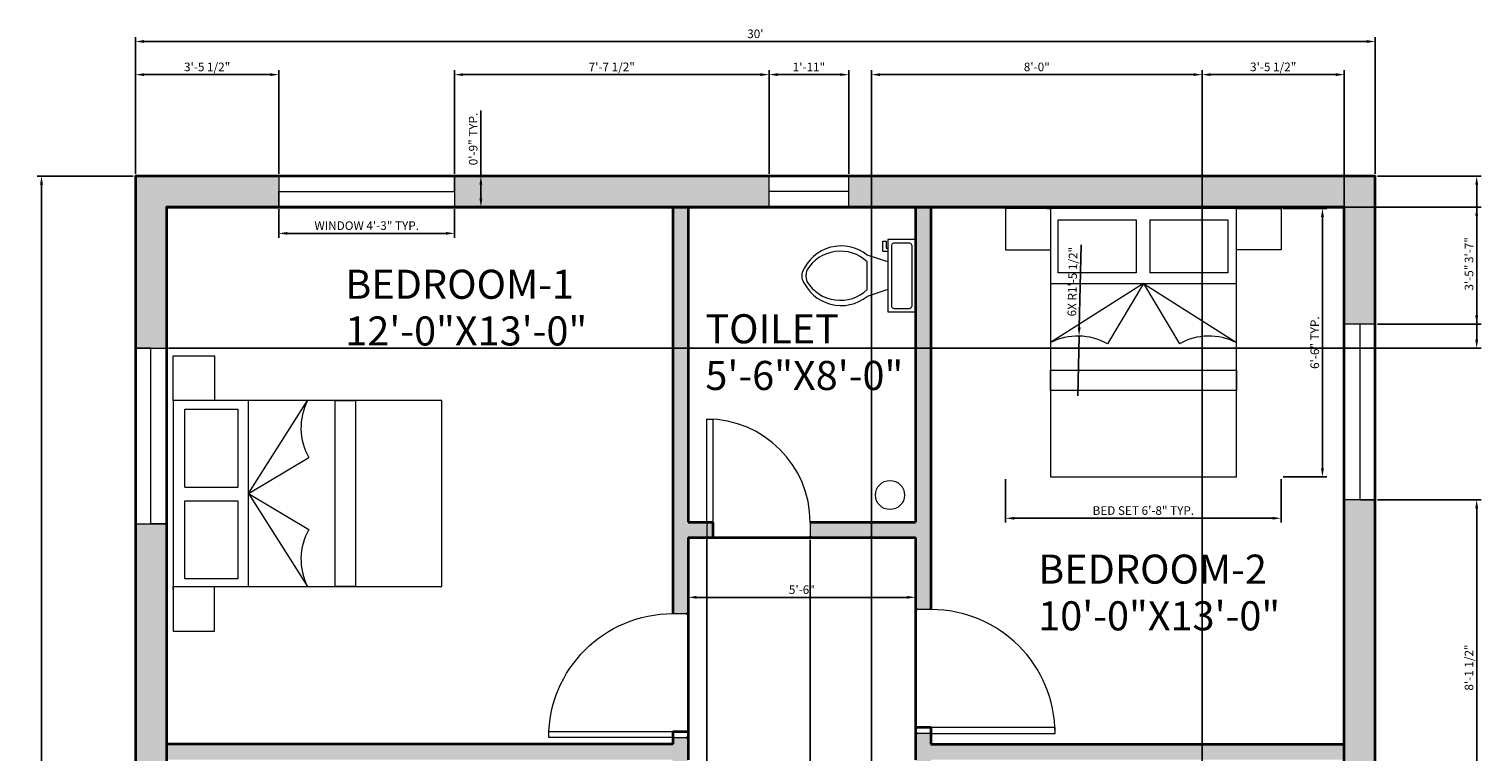
# Model space of a CAD drawing. Units: inches. Extents: x 10 to 434, y 91 to 681.
# Tile 2 of 2: x 12 to 434, y 471 to 681. Entities that reach past the tile are written whole.
import ezdxf

# ---------------------------------------------------------------- set-up
doc = ezdxf.new("R2010")
doc.units = ezdxf.units.IN
for name, color, linetype, lineweight in [('A-ANNO-DIMS', 2, 'Continuous', 18), ('A-AREA-IDEN', 7, 'Continuous', 18), ('A-DOOR', 4, 'Continuous', 18), ('A-FLOR-FIXT', 9, 'Continuous', 18), ('A-FURN', 8, 'Continuous', 18), ('A-GLAZ', 4, 'Continuous', 18), ('A-WALL', 7, 'Continuous', 35), ('A-WALL-PATT', 251, 'Continuous', 13)]:
    doc.layers.add(name, color=color, linetype=linetype, lineweight=lineweight)
doc.styles.get("Standard").update_dxf_attribs({"font": 'arial.ttf'})
doc.dimstyles.new('ISO-25', dxfattribs={"dimtxt": 2.5, "dimasz": 2.5, "dimexe": 1.25, "dimexo": 0.625, "dimtad": 1, "dimlunit": 3, "dimtxsty": 'Standard', "dimcen": 2.5, "dimadec": 0, "dimazin": 0, "dimtfac": 1, "dimtmove": 0, "dimatfit": 3, "dimfxl": 1, "dimarcsym": 0})

# ---------------------------------------------------------------- blocks, each defined once
blk = doc.blocks.new('*U4')
for p, q in [((0, 0), (0, -4)), ((-36, 0), (-36, -4))]:
    blk.add_line(p, q)
blk.add_lwpolyline([(0, 0), (0, 36), (-1.75, 36), (-1.75, 0)], close=True)
blk.add_arc((0, 0), 36, 90, 180)
blk = doc.blocks.new('*U3')
for p, q in [((0, 0), (0, -4)), ((30, 0), (30, -4))]:
    blk.add_line(p, q)
blk.add_lwpolyline([(0, 0), (0, 30), (1.75, 30), (1.75, 0)], close=True)
blk.add_arc((0, 0), 30, 0, 90)
blk = doc.blocks.new('*U7')
for p, q in [((9.5, -6), (9.5, -2)), ((-8, -8.5), (-8, -8)), ((-7, -8), (-7, -9.5)), ((-4, -8), (-6, -14)), ((4, -8), (6, -14)), ((-10, -8.5), (-8, -8.5)), ((-10, -9.5), (-10, -8.5)), ((-7, -9.5), (-10, -9.5)), ((4, -14), (-4, -14))]:
    blk.add_line(p, q)
blk.add_lwpolyline([(10.5, -8), (10.5, 0), (-10.5, 0), (-10.5, -8)], close=True)
for points in [[(-9.5, -2), (-9.5, -6)], [(8.5, -1), (-8.5, -1)], [(-8.5, -7), (8.5, -7)]]:
    blk.add_lwpolyline(points)
for centre, radius, start, end in [((-8.62, -1.88), 0.884, 81.8699, 188.1301), ((8.62, -1.88), 0.884, 351.8699, 98.1301), ((-8.62, -6.12), 0.884, 171.8699, 278.1301), ((8.62, -6.12), 0.884, 261.8699, 8.1301), ((3.52, -21.58), 12.17, 141.4691, 247.9714), ((4.2, -21.82), 11.33, 136.3677, 238.9468), ((-3.52, -21.58), 12.17, 292.0284, 38.5307), ((-4.2, -21.82), 11.33, 301.053, 43.6321), ((0, -27.88), 4, 245.7318, 294.2682), ((0, -29), 4, 254.8605, 285.1395)]:
    blk.add_arc(centre, radius, start, end)
blk = doc.blocks.new('*D11')
at = {"layer": 'A-ANNO-DIMS', "color": 0, "lineweight": -2, "transparency": 16777216}
for p, q in [((42.44, 638.74), (14.54, 638.74)), ((15.79, 636.24), (15.79, 161.24)), ((42.44, 158.74), (14.54, 158.74))]:
    blk.add_line(p, q, dxfattribs=at)
at = {"layer": 'A-ANNO-DIMS', "color": 0, "transparency": 16777216}
for points in [[(15.37, 636.24), (16.21, 636.24), (15.79, 638.74)], [(15.37, 161.24), (16.21, 161.24), (15.79, 158.74)]]:
    blk.add_solid(points, dxfattribs=at)
at = {"layer": 'Defpoints', "color": 0, "transparency": 16777216}
for p in [(43.07, 638.74), (15.79, 158.74), (43.07, 158.74)]:
    blk.add_point(p, dxfattribs=at)
at = {"layer": 'A-ANNO-DIMS', "color": 0, "transparency": 16777216, "insert": (13.89, 398.74), "char_height": 2.5, "attachment_point": 5, "rotation": 90}
blk.add_mtext("40'", dxfattribs=at)
blk = doc.blocks.new('*D12')
at = {"layer": 'A-ANNO-DIMS', "color": 0, "lineweight": -2, "transparency": 16777216}
for p, q in [((43.07, 639.37), (43.07, 679.06)), ((400.57, 677.81), (45.57, 677.81)), ((403.07, 639.37), (403.07, 679.06))]:
    blk.add_line(p, q, dxfattribs=at)
at = {"layer": 'A-ANNO-DIMS', "color": 0, "transparency": 16777216}
for points in [[(45.57, 678.23), (45.57, 677.4), (43.07, 677.81)], [(400.57, 678.23), (400.57, 677.4), (403.07, 677.81)]]:
    blk.add_solid(points, dxfattribs=at)
at = {"layer": 'Defpoints', "color": 0, "transparency": 16777216}
for p in [(43.07, 677.81), (43.07, 638.74), (403.07, 638.74)]:
    blk.add_point(p, dxfattribs=at)
at = {"layer": 'A-ANNO-DIMS', "color": 0, "transparency": 16777216, "insert": (223.07, 679.72), "char_height": 2.5, "attachment_point": 5}
blk.add_mtext("30'", dxfattribs=at)
blk = doc.blocks.new('*D14')
at = {"layer": 'A-ANNO-DIMS', "color": 0, "lineweight": -2, "transparency": 16777216}
for p, q in [((203.57, 533.12), (203.57, 515.14)), ((269.57, 533.12), (269.57, 515.14)), ((206.07, 516.39), (267.07, 516.39))]:
    blk.add_line(p, q, dxfattribs=at)
at = {"layer": 'A-ANNO-DIMS', "color": 0, "transparency": 16777216}
for points in [[(206.07, 516.81), (206.07, 515.98), (203.57, 516.39)], [(267.07, 516.81), (267.07, 515.98), (269.57, 516.39)]]:
    blk.add_solid(points, dxfattribs=at)
at = {"layer": 'Defpoints', "color": 0, "transparency": 16777216}
for p in [(203.57, 533.74), (269.57, 533.74), (269.57, 516.39)]:
    blk.add_point(p, dxfattribs=at)
at = {"layer": 'A-ANNO-DIMS', "color": 0, "transparency": 16777216, "insert": (236.57, 518.29), "char_height": 2.5, "attachment_point": 5}
blk.add_mtext('5\'-6"', dxfattribs=at)
blk = doc.blocks.new('BED-DOUBLE-WITH-NIGHTSTANDS')
for p, q in [((40, 21.85), (13, 39)), ((40, 21.85), (29.54, 39.37)), ((40, 21.85), (50.46, 39.37)), ((40, 21.85), (67, 39)), ((67, 21.85), (13, 21.85)), ((38.13, 3.34), (38.13, 18.76)), ((42.13, 3.34), (42.13, 18.76)), ((0, 0), (0, 12)), ((0, 12), (13, 12)), ((68, 12), (67, 12)), ((80, 12), (68, 12)), ((80, 0), (80, 12)), ((1, 0), (0, 0)), ((13, 0), (1, 0)), ((68, 0), (80, 0))]:
    blk.add_line(p, q)
for points in [[(67, 78), (13, 78), (13, 0), (67, 0)], [(67, 46.98), (13, 46.98), (13, 52.9), (67, 52.9)], [(67, 0), (68, 0), (68, 0), (67, 0)]]:
    blk.add_lwpolyline(points, close=True)
for points in [[(38.13, 3.34), (15.5, 3.34), (15.5, 18.76), (38.13, 18.76)], [(42.13, 18.76), (64.76, 18.76), (64.76, 3.34), (42.13, 3.34)]]:
    blk.add_lwpolyline(points)
for centre, start, end in [((20.93, 54.43), 242.8058, 299.7512), ((59.07, 54.43), 240.2488, 297.1942)]:
    blk.add_arc(centre, 17.35, start, end)
blk = doc.blocks.new('WINDOW-51IN')
for p, q in [((0, 9), (0, 0)), ((51, 4.5), (51, 9)), ((51, 9), (51, 0)), ((0, 0), (0, 4.5)), ((0, 4.5), (51, 4.5))]:
    blk.add_line(p, q)
blk = doc.blocks.new('*D20')
at = {"layer": 'A-ANNO-DIMS', "color": 0, "lineweight": -2, "transparency": 16777216}
for p, q in [((84.72, 629.12), (84.72, 620.84)), ((135.72, 629.12), (135.72, 620.84)), ((87.22, 622.09), (133.22, 622.09))]:
    blk.add_line(p, q, dxfattribs=at)
at = {"layer": 'A-ANNO-DIMS', "color": 0, "transparency": 16777216}
for points in [[(87.22, 622.51), (87.22, 621.68), (84.72, 622.09)], [(133.22, 622.51), (133.22, 621.68), (135.72, 622.09)]]:
    blk.add_solid(points, dxfattribs=at)
at = {"layer": 'Defpoints', "color": 0, "transparency": 16777216}
for p in [(84.72, 629.74), (135.72, 629.74), (135.72, 622.09)]:
    blk.add_point(p, dxfattribs=at)
at = {"layer": 'A-ANNO-DIMS', "color": 0, "transparency": 16777216, "insert": (110.22, 624.01), "char_height": 2.5, "attachment_point": 5}
blk.add_mtext('WINDOW 4\'-3" TYP.', dxfattribs=at)
blk = doc.blocks.new('*D21')
at = {"layer": 'A-ANNO-DIMS', "color": 0, "lineweight": -2, "transparency": 16777216}
for p, q in [((143.37, 638.74), (143.37, 657.73)), ((136.34, 638.74), (144.62, 638.74)), ((143.37, 632.24), (143.37, 636.24)), ((136.34, 629.74), (144.62, 629.74))]:
    blk.add_line(p, q, dxfattribs=at)
at = {"layer": 'A-ANNO-DIMS', "color": 0, "transparency": 16777216}
for points in [[(142.95, 636.24), (143.78, 636.24), (143.37, 638.74)], [(142.95, 632.24), (143.78, 632.24), (143.37, 629.74)]]:
    blk.add_solid(points, dxfattribs=at)
at = {"layer": 'Defpoints', "color": 0, "transparency": 16777216}
for p in [(135.72, 638.74), (143.37, 638.74), (135.72, 629.74)]:
    blk.add_point(p, dxfattribs=at)
at = {"layer": 'A-ANNO-DIMS', "color": 0, "transparency": 16777216, "insert": (141.46, 649.49), "char_height": 2.5, "attachment_point": 5, "rotation": 90}
blk.add_mtext('0\'-9" TYP.', dxfattribs=at)
blk = doc.blocks.new('*D22')
at = {"layer": 'A-ANNO-DIMS', "color": 0, "lineweight": -2, "transparency": 16777216}
for p, q in [((295.73, 550.73), (295.73, 538.1)), ((375.73, 550.73), (375.73, 538.1)), ((373.23, 539.35), (298.23, 539.35))]:
    blk.add_line(p, q, dxfattribs=at)
at = {"layer": 'A-ANNO-DIMS', "color": 0, "transparency": 16777216}
for points in [[(298.23, 539.77), (298.23, 538.94), (295.73, 539.35)], [(373.23, 539.77), (373.23, 538.94), (375.73, 539.35)]]:
    blk.add_solid(points, dxfattribs=at)
at = {"layer": 'Defpoints', "color": 0, "transparency": 16777216}
for p in [(295.73, 551.35), (375.73, 551.35), (295.73, 539.35)]:
    blk.add_point(p, dxfattribs=at)
at = {"layer": 'A-ANNO-DIMS', "color": 0, "transparency": 16777216, "insert": (335.73, 541.27), "char_height": 2.5, "attachment_point": 5}
blk.add_mtext('BED SET 6\'-8" TYP.', dxfattribs=at)
blk = doc.blocks.new('*D23')
at = {"layer": 'A-ANNO-DIMS', "color": 0, "lineweight": -2, "transparency": 16777216}
for p, q in [((376.36, 629.35), (388.98, 629.35)), ((387.73, 626.85), (387.73, 553.85)), ((376.36, 551.35), (388.98, 551.35))]:
    blk.add_line(p, q, dxfattribs=at)
at = {"layer": 'A-ANNO-DIMS', "color": 0, "transparency": 16777216}
for points in [[(387.31, 626.85), (388.15, 626.85), (387.73, 629.35)], [(387.31, 553.85), (388.15, 553.85), (387.73, 551.35)]]:
    blk.add_solid(points, dxfattribs=at)
at = {"layer": 'Defpoints', "color": 0, "transparency": 16777216}
for p in [(375.73, 629.35), (375.73, 551.35), (387.73, 551.35)]:
    blk.add_point(p, dxfattribs=at)
at = {"layer": 'A-ANNO-DIMS', "color": 0, "transparency": 16777216, "insert": (385.83, 590.35), "char_height": 2.5, "attachment_point": 5, "rotation": 90}
blk.add_mtext('6\'-6" TYP.', dxfattribs=at)
blk = doc.blocks.new('*D27')
at = {"layer": 'A-ANNO-DIMS', "color": 0, "lineweight": -2, "transparency": 16777216}
for p, q in [((352.79, 283.87), (352.79, 669.44)), ((355.29, 668.19), (391.57, 668.19)), ((394.07, 283.87), (394.07, 669.44))]:
    blk.add_line(p, q, dxfattribs=at)
at = {"layer": 'A-ANNO-DIMS', "color": 0, "transparency": 16777216}
for points in [[(355.29, 668.61), (355.29, 667.78), (352.79, 668.19)], [(391.57, 668.61), (391.57, 667.78), (394.07, 668.19)]]:
    blk.add_solid(points, dxfattribs=at)
at = {"layer": 'Defpoints', "color": 0, "transparency": 16777216}
for p in [(394.07, 668.19), (352.79, 283.24), (394.07, 283.24)]:
    blk.add_point(p, dxfattribs=at)
at = {"layer": 'A-ANNO-DIMS', "color": 0, "transparency": 16777216, "insert": (373.43, 670.11), "char_height": 2.5, "attachment_point": 5}
blk.add_mtext('3\'-5 1/2"', dxfattribs=at)
blk = doc.blocks.new('*D28')
at = {"layer": 'A-ANNO-DIMS', "color": 0, "lineweight": -2, "transparency": 16777216}
for p, q in [((256.79, 283.87), (256.79, 669.44)), ((259.29, 668.19), (350.29, 668.19)), ((352.79, 283.87), (352.79, 669.44))]:
    blk.add_line(p, q, dxfattribs=at)
at = {"layer": 'A-ANNO-DIMS', "color": 0, "transparency": 16777216}
for points in [[(259.29, 668.61), (259.29, 667.78), (256.79, 668.19)], [(350.29, 668.61), (350.29, 667.78), (352.79, 668.19)]]:
    blk.add_solid(points, dxfattribs=at)
at = {"layer": 'Defpoints', "color": 0, "transparency": 16777216}
for p in [(352.79, 668.19), (256.79, 283.24), (352.79, 283.24)]:
    blk.add_point(p, dxfattribs=at)
at = {"layer": 'A-ANNO-DIMS', "color": 0, "transparency": 16777216, "insert": (304.79, 670.1), "char_height": 2.5, "attachment_point": 5}
blk.add_mtext('8\'-0"', dxfattribs=at)
blk = doc.blocks.new('*D29')
at = {"layer": 'A-ANNO-DIMS', "color": 0, "lineweight": -2, "transparency": 16777216}
for p, q in [((43.07, 639.37), (43.07, 669.44)), ((45.57, 668.19), (82.22, 668.19)), ((84.72, 639.37), (84.72, 669.44))]:
    blk.add_line(p, q, dxfattribs=at)
at = {"layer": 'A-ANNO-DIMS', "color": 0, "transparency": 16777216}
for points in [[(45.57, 668.61), (45.57, 667.78), (43.07, 668.19)], [(82.22, 668.61), (82.22, 667.78), (84.72, 668.19)]]:
    blk.add_solid(points, dxfattribs=at)
at = {"layer": 'Defpoints', "color": 0, "transparency": 16777216}
for p in [(84.72, 668.19), (43.07, 638.74), (84.72, 638.74)]:
    blk.add_point(p, dxfattribs=at)
at = {"layer": 'A-ANNO-DIMS', "color": 0, "transparency": 16777216, "insert": (63.89, 670.11), "char_height": 2.5, "attachment_point": 5}
blk.add_mtext('3\'-5 1/2"', dxfattribs=at)
blk = doc.blocks.new('*D30')
at = {"layer": 'A-ANNO-DIMS', "color": 0, "lineweight": -2, "transparency": 16777216}
for p, q in [((135.72, 639.37), (135.72, 669.44)), ((138.22, 668.19), (224.54, 668.19)), ((227.04, 639.37), (227.04, 669.44))]:
    blk.add_line(p, q, dxfattribs=at)
at = {"layer": 'A-ANNO-DIMS', "color": 0, "transparency": 16777216}
for points in [[(138.22, 668.61), (138.22, 667.78), (135.72, 668.19)], [(224.54, 668.61), (224.54, 667.78), (227.04, 668.19)]]:
    blk.add_solid(points, dxfattribs=at)
at = {"layer": 'Defpoints', "color": 0, "transparency": 16777216}
for p in [(227.04, 668.19), (135.72, 638.74), (227.04, 638.74)]:
    blk.add_point(p, dxfattribs=at)
at = {"layer": 'A-ANNO-DIMS', "color": 0, "transparency": 16777216, "insert": (181.38, 670.11), "char_height": 2.5, "attachment_point": 5}
blk.add_mtext('7\'-7 1/2"', dxfattribs=at)
blk = doc.blocks.new('*D31')
at = {"layer": 'A-ANNO-DIMS', "color": 0, "lineweight": -2, "transparency": 16777216}
for p, q in [((227.04, 639.37), (227.04, 669.44)), ((229.54, 668.19), (247.7, 668.19)), ((250.2, 639.37), (250.2, 669.44))]:
    blk.add_line(p, q, dxfattribs=at)
at = {"layer": 'A-ANNO-DIMS', "color": 0, "transparency": 16777216}
for points in [[(229.54, 668.61), (229.54, 667.78), (227.04, 668.19)], [(247.7, 668.61), (247.7, 667.78), (250.2, 668.19)]]:
    blk.add_solid(points, dxfattribs=at)
at = {"layer": 'Defpoints', "color": 0, "transparency": 16777216}
for p in [(250.2, 668.19), (227.04, 638.74), (250.2, 638.74)]:
    blk.add_point(p, dxfattribs=at)
at = {"layer": 'A-ANNO-DIMS', "color": 0, "transparency": 16777216, "insert": (238.62, 670.07), "char_height": 2.5, "attachment_point": 5}
blk.add_mtext('1\'-11"', dxfattribs=at)
blk = doc.blocks.new('*D34')
at = {"layer": 'A-ANNO-DIMS', "color": 0, "lineweight": -2, "transparency": 16777216}
for p, q in [((52.69, 629.74), (433.77, 629.74)), ((432.52, 591.23), (432.52, 627.24)), ((52.69, 588.73), (433.77, 588.73))]:
    blk.add_line(p, q, dxfattribs=at)
at = {"layer": 'A-ANNO-DIMS', "color": 0, "transparency": 16777216}
for points in [[(432.1, 627.24), (432.93, 627.24), (432.52, 629.74)], [(432.1, 591.23), (432.93, 591.23), (432.52, 588.73)]]:
    blk.add_solid(points, dxfattribs=at)
at = {"layer": 'Defpoints', "color": 0, "transparency": 16777216}
for p in [(52.07, 629.74), (432.52, 629.74), (52.07, 588.73)]:
    blk.add_point(p, dxfattribs=at)
at = {"layer": 'A-ANNO-DIMS', "color": 0, "transparency": 16777216, "insert": (430.61, 609.24), "char_height": 2.5, "attachment_point": 5, "rotation": 90}
blk.add_mtext('3\'-5"', dxfattribs=at)
blk = doc.blocks.new('*D35')
at = {"layer": 'A-ANNO-DIMS', "color": 0, "lineweight": -2, "transparency": 16777216}
for p, q in [((403.69, 638.74), (433.77, 638.74)), ((432.52, 636.24), (432.52, 598.24)), ((403.69, 595.74), (433.77, 595.74))]:
    blk.add_line(p, q, dxfattribs=at)
at = {"layer": 'A-ANNO-DIMS', "color": 0, "transparency": 16777216}
for points in [[(432.1, 636.24), (432.93, 636.24), (432.52, 638.74)], [(432.1, 598.24), (432.93, 598.24), (432.52, 595.74)]]:
    blk.add_solid(points, dxfattribs=at)
at = {"layer": 'Defpoints', "color": 0, "transparency": 16777216}
for p in [(403.07, 638.74), (403.07, 595.74), (432.52, 595.74)]:
    blk.add_point(p, dxfattribs=at)
at = {"layer": 'A-ANNO-DIMS', "color": 0, "transparency": 16777216, "insert": (430.61, 617.24), "char_height": 2.5, "attachment_point": 5, "rotation": 90}
blk.add_mtext('3\'-7"', dxfattribs=at)
blk = doc.blocks.new('*D36')
at = {"layer": 'A-ANNO-DIMS', "color": 0, "lineweight": -2, "transparency": 16777216}
for p, q in [((403.69, 544.74), (433.77, 544.74)), ((432.52, 542.24), (432.52, 449.76)), ((403.69, 447.26), (433.77, 447.26))]:
    blk.add_line(p, q, dxfattribs=at)
at = {"layer": 'A-ANNO-DIMS', "color": 0, "transparency": 16777216}
for points in [[(432.1, 542.24), (432.93, 542.24), (432.52, 544.74)], [(432.1, 449.76), (432.93, 449.76), (432.52, 447.26)]]:
    blk.add_solid(points, dxfattribs=at)
at = {"layer": 'Defpoints', "color": 0, "transparency": 16777216}
for p in [(403.07, 544.74), (403.07, 447.26), (432.52, 447.26)]:
    blk.add_point(p, dxfattribs=at)
at = {"layer": 'A-ANNO-DIMS', "color": 0, "transparency": 16777216, "insert": (430.6, 496), "char_height": 2.5, "attachment_point": 5, "rotation": 90}
blk.add_mtext('8\'-1 1/2"', dxfattribs=at)
blk = doc.blocks.new('*D40')
at = {"layer": 'A-ANNO-DIMS', "color": 0, "lineweight": -2, "transparency": 16777216}
for p, q in [((208.98, 533.52), (208.98, 92.04)), ((238.98, 533.12), (238.98, 92.04)), ((211.48, 93.29), (236.48, 93.29))]:
    blk.add_line(p, q, dxfattribs=at)
at = {"layer": 'A-ANNO-DIMS', "color": 0, "transparency": 16777216}
for points in [[(211.48, 93.71), (211.48, 92.88), (208.98, 93.29)], [(236.48, 93.71), (236.48, 92.88), (238.98, 93.29)]]:
    blk.add_solid(points, dxfattribs=at)
at = {"layer": 'Defpoints', "color": 0, "transparency": 16777216}
for p in [(208.98, 534.14), (238.98, 533.74), (238.98, 93.29)]:
    blk.add_point(p, dxfattribs=at)
at = {"layer": 'A-ANNO-DIMS', "color": 0, "transparency": 16777216, "insert": (223.98, 95.2), "char_height": 2.5, "attachment_point": 5}
blk.add_mtext('2\'-6"', dxfattribs=at)
blk = doc.blocks.new('*D44')
at = {"layer": 'A-ANNO-DIMS', "color": 0, "lineweight": -2, "transparency": 16777216}
for p, q in [((317.64, 618.76), (317.1, 594.77)), ((316.66, 574.92), (317.05, 592.27))]:
    blk.add_line(p, q, dxfattribs=at)
at = {"layer": 'A-ANNO-DIMS', "color": 0, "transparency": 16777216}
blk.add_solid([(316.69, 594.78), (317.52, 594.76), (317.05, 592.27)], dxfattribs=at)
at = {"layer": 'Defpoints', "color": 0, "transparency": 16777216}
for p in [(317.05, 592.27), (316.66, 574.92)]:
    blk.add_point(p, dxfattribs=at)
at = {"layer": 'A-ANNO-DIMS', "color": 0, "transparency": 16777216, "insert": (315.48, 608.06), "char_height": 2.5, "attachment_point": 5, "rotation": 88.723}
blk.add_mtext('6X R1\'-5 1/2"', dxfattribs=at)

msp = doc.modelspace()

# ---------------------------------------------------------------- hatches: boundary and pattern name
at = {"layer": 'A-WALL-PATT'}
h = msp.add_hatch(color=256, dxfattribs=at)
h.dxf.hatch_style = 1
h.paths.add_polyline_path([(84.716, 634.244), (84.716, 638.744), (43.066, 638.744), (43.066, 588.73), (47.566, 588.73), (52.066, 588.73), (52.066, 629.744), (84.716, 629.744)])
h.paths.add_polyline_path([(227.044, 638.744), (135.716, 638.744), (135.716, 629.744), (227.044, 629.744)])
h.paths.add_polyline_path([(52.066, 537.73), (43.066, 537.73), (43.066, 432.018), (52.066, 432.018)])
h.paths.add_polyline_path([(52.066, 381.018), (43.066, 381.018), (43.066, 289.264), (47.566, 289.264), (52.066, 289.264)])
h.paths.add_polyline_path([(52.066, 238.264), (43.066, 238.264), (43.066, 158.744), (97.573, 158.744), (97.573, 163.244), (97.573, 167.744), (52.066, 167.744)])
h.paths.add_polyline_path([(207.929, 163.896), (207.929, 167.744), (148.573, 167.744), (148.573, 158.744), (207.929, 158.744)])
h.paths.add_polyline_path([(403.066, 316.579), (394.066, 316.579), (394.066, 167.744), (243.929, 167.744), (243.929, 163.896), (243.929, 158.744), (403.066, 158.744)])
h.paths.add_polyline_path([(403.066, 405.259), (398.566, 405.259), (394.066, 405.259), (394.066, 358.579), (403.066, 358.579)])
h.paths.add_polyline_path([(394.066, 473.744), (274.066, 473.744), (274.066, 476.846), (270.089, 476.846), (269.566, 476.846), (269.566, 469.244), (394.066, 469.244)])
h.paths.add_polyline_path([(203.566, 475.661), (203.066, 475.661), (199.066, 475.661), (199.066, 473.744), (52.066, 473.744), (52.066, 469.244), (199.066, 469.244), (199.066, 466.04), (202.989, 466.04), (203.566, 466.04), (203.566, 469.244)])
h.paths.add_polyline_path([(203.566, 426.04), (202.989, 426.04), (199.066, 426.04), (199.066, 329.744), (184.066, 329.744), (52.066, 329.744), (52.066, 325.244), (184.066, 325.244), (203.566, 325.244)])
h.paths.add_polyline_path([(201.066, 283.244), (202.066, 283.244), (214.742, 283.244), (214.742, 283.768), (214.742, 287.744), (202.066, 287.744), (196.566, 287.744), (196.566, 167.744), (201.066, 167.744)])
h.paths.add_polyline_path([(394.066, 287.744), (250.742, 287.744), (250.742, 283.768), (250.742, 283.244), (394.066, 283.244)], flags=17)
h.paths.add_polyline_path([(394.066, 369.085), (370.066, 369.085), (365.066, 369.085), (365.066, 364.585), (394.066, 364.585)])
h.paths.add_polyline_path([(274.066, 469.244), (269.566, 469.244), (269.566, 440.244), (274.066, 440.244)])
h.paths.add_polyline_path([(403.066, 544.736), (394.066, 544.736), (394.066, 447.259), (403.066, 447.259)])
h.paths.add_polyline_path([(206.394, 574.303), (265.532, 574.303), (265.532, 587.233), (206.394, 587.233)], flags=9)
h.paths.add_polyline_path([(206.366, 587.835), (252.012, 587.835), (252.012, 600.937), (206.366, 600.937)], flags=9)
h.paths.add_polyline_path([(303.038, 504.495), (375.295, 504.495), (375.295, 517.433), (303.038, 517.433)], flags=9)
h.paths.add_polyline_path([(303.011, 518.033), (378.795, 518.033), (378.795, 531.136), (303.011, 531.136)], flags=9)
h = msp.add_hatch(color=256, dxfattribs=at)
h.dxf.hatch_style = 1
h.paths.add_polyline_path([(403.066, 638.744), (250.195, 638.744), (250.195, 629.744), (269.566, 629.744), (394.066, 629.744), (394.066, 595.736), (403.066, 595.736)])
h.paths.add_polyline_path([(203.566, 629.744), (199.066, 629.744), (199.066, 533.744), (199.066, 511.661), (203.066, 511.661), (203.566, 511.661), (203.566, 533.744), (210.73, 533.744), (210.73, 538.144), (208.98, 538.144), (203.566, 538.244)])
h.paths.add_polyline_path([(274.066, 629.744), (269.566, 629.744), (269.566, 538.244), (238.98, 538.244), (238.98, 534.144), (238.98, 533.744), (269.566, 533.744), (269.566, 512.846), (270.089, 512.846), (274.066, 512.846)])

# ---------------------------------------------------------------- linework, layer by layer
at = {"layer": 'A-FLOR-FIXT'}
msp.add_circle((262.162, 546.101), 4.228, dxfattribs=at)
at = {"layer": 'A-GLAZ'}
for p, q in [((227.044, 629.744), (227.044, 638.744)), ((250.195, 629.744), (250.195, 638.744)), ((250.195, 634.244), (227.044, 634.244)), ((403.066, 595.736), (394.066, 595.736)), ((398.566, 595.736), (398.566, 544.736)), ((403.066, 544.736), (394.066, 544.736)), ((398.566, 544.736), (403.066, 544.736))]:
    msp.add_line(p, q, dxfattribs=at)
at = {"layer": 'A-WALL'}
for p, q in [((52.066, 629.744), (394.066, 629.744)), ((199.066, 629.744), (199.066, 533.744)), ((269.566, 629.744), (203.566, 629.744)), ((203.566, 629.744), (203.566, 538.244)), ((269.566, 629.744), (269.566, 538.244)), ((394.066, 629.744), (274.066, 629.744)), ((274.066, 629.744), (274.066, 512.846)), ((203.566, 538.244), (210.73, 538.244)), ((210.73, 538.144), (210.73, 533.744)), ((238.979, 538.244), (269.566, 538.244)), ((199.066, 533.744), (199.066, 511.661)), ((203.566, 533.744), (269.566, 533.744)), ((203.566, 533.744), (203.566, 469.244)), ((238.98, 534.144), (238.98, 533.744)), ((269.566, 533.744), (269.566, 469.244)), ((203.066, 511.661), (203.566, 511.661)), ((270.089, 512.846), (269.566, 512.846)), ((199.066, 477.411), (199.066, 473.744)), ((199.066, 477.411), (203.566, 477.411)), ((274.089, 478.596), (269.566, 478.596)), ((274.066, 478.596), (274.066, 473.744)), ((199.066, 473.744), (52.066, 473.744)), ((203.066, 475.661), (203.566, 475.661)), ((270.089, 476.846), (269.566, 476.846)), ((274.066, 473.744), (394.066, 473.744))]:
    msp.add_line(p, q, dxfattribs=at)
msp.add_lwpolyline([(43.066, 158.744), (403.066, 158.744), (403.066, 638.744), (43.066, 638.744)], close=True, dxfattribs=at)
msp.add_lwpolyline([(243.929, 167.744), (394.066, 167.744), (394.066, 629.744), (52.066, 629.744), (52.066, 167.744), (207.929, 167.744)], dxfattribs=at)

# ---------------------------------------------------------------- block references
at = {"layer": 'A-DOOR'}
msp.add_blockref('*U3', (208.98, 538.144), dxfattribs=at)
at = {"layer": 'A-DOOR', "xscale": -1, "rotation": 90}
msp.add_blockref('*U4', (199.066, 475.661), dxfattribs=at)
at = {"layer": 'A-DOOR', "rotation": 270}
msp.add_blockref('*U4', (274.089, 476.846), dxfattribs=at)
at = {"layer": 'A-FLOR-FIXT', "rotation": 270}
msp.add_blockref('*U7', (269.566, 609.786), dxfattribs=at)
at = {"layer": 'A-FURN'}
for p, rotation in [((375.732, 629.354), 180), ((54.056, 586.527), 270.0000000000005)]:
    msp.add_blockref('BED-DOUBLE-WITH-NIGHTSTANDS', p, dxfattribs=dict(at, rotation=rotation))
at = {"layer": 'A-GLAZ'}
msp.add_blockref('WINDOW-51IN', (84.716, 629.744), dxfattribs=at)
at = {"layer": 'A-GLAZ', "rotation": 90.00000000000031}
msp.add_blockref('WINDOW-51IN', (52.065, 537.73), dxfattribs=at)

# ---------------------------------------------------------------- texts
at = {"layer": 'A-AREA-IDEN'}
for s, height, p in [('BEDROOM-1', 8.4412, (103.996, 603.089)), ('12\'-0"X13\'-0"', 8.44119, (103.996, 589.529)), ('TOILET', 8.4412, (208.549, 590.162)), ('5\'-6"X8\'-0"', 8.44119, (208.549, 576.602)), ('BEDROOM-2', 8.4412, (305.195, 520.361)), ('10\'-0"X13\'-0"', 8.44119, (305.195, 506.801))]:
    msp.add_text(s, height=height, dxfattribs=at).set_placement(p)

# ---------------------------------------------------------------- dimensions: what is measured, and where the dimension line sits
at = {"layer": 'A-ANNO-DIMS'}
for base, p1, p2, override, picture, middle in [((43.066, 677.815), (403.066, 638.744), (43.066, 638.744), {"dimclrd": 0, "dimclre": 0, "dimclrt": 0}, '*D12', (223.066, 679.717)), ((84.7156, 668.1937), (43.0657, 638.7437), (84.7156, 638.7437), {"dimdec": 1, "dimlfac": 1, "dimrnd": 0, "dimzin": 1, "dimdsep": 46, "dimlunit": 4, "dimfrac": 2}, '*D29', (63.8907, 670.1122)), ((227.044, 668.194), (135.716, 638.744), (227.044, 638.744), {"dimdec": 1, "dimlfac": 1, "dimrnd": 0, "dimzin": 1, "dimdsep": 46, "dimlunit": 4, "dimfrac": 2}, '*D30', (181.38, 670.111)), ((250.195, 668.194), (227.044, 638.744), (250.195, 638.744), {"dimdec": 1, "dimlfac": 1, "dimrnd": 0, "dimzin": 1, "dimdsep": 46, "dimlunit": 4, "dimfrac": 2}, '*D31', (238.62, 670.074)), ((352.787, 668.194), (256.787, 283.244), (352.787, 283.244), {"dimdec": 1, "dimlfac": 1, "dimrnd": 0, "dimzin": 1, "dimdsep": 46, "dimlunit": 4, "dimfrac": 2}, '*D28', (304.787, 670.095)), ((394.066, 668.194), (352.787, 283.244), (394.066, 283.244), {"dimdec": 1, "dimlfac": 1, "dimrnd": 0, "dimzin": 1, "dimdsep": 46, "dimlunit": 4, "dimfrac": 2}, '*D27', (373.426, 670.112)), ((269.566, 516.392), (203.566, 533.744), (269.566, 533.744), {"dimclrd": 0, "dimclre": 0, "dimclrt": 0}, '*D14', (236.566, 518.293)), ((238.98, 93.294), (208.98, 534.144), (238.98, 533.744), {"dimdec": 1, "dimlfac": 1, "dimrnd": 0, "dimzin": 1, "dimdsep": 46, "dimlunit": 4, "dimfrac": 2}, '*D40', (223.98, 95.195))]:
    dim = msp.add_linear_dim(base=base, p1=p1, p2=p2, dimstyle='ISO-25', override=override, dxfattribs=at)
    dim.commit()
    dim.dimension.update_dxf_attribs({"geometry": picture, "text_midpoint": middle})
for base, p1, p2, angle, text, picture, middle in [((143.366, 638.744), (135.716, 629.744), (135.716, 638.744), 90, '<> TYP.', '*D21', (141.464, 649.488)), ((387.731, 551.354), (375.731, 629.354), (375.731, 551.354), 270, '<> TYP.', '*D23', (385.83, 590.354)), ((295.731, 539.354), (375.731, 551.354), (295.731, 551.354), 180, 'BED SET <> TYP.', '*D22', (335.731, 541.271))]:
    dim = msp.add_linear_dim(base=base, p1=p1, p2=p2, angle=angle, text=text, dimstyle='ISO-25', override={"dimdec": 1, "dimlfac": 1, "dimrnd": 0, "dimzin": 1, "dimdsep": 46, "dimlunit": 4, "dimfrac": 2}, dxfattribs=at)
    dim.commit()
    dim.dimension.update_dxf_attribs({"geometry": picture, "text_midpoint": middle})
for base, p1, p2, override, picture, middle in [((15.79, 158.744), (43.066, 638.744), (43.066, 158.744), {"dimclrd": 0, "dimclre": 0, "dimclrt": 0}, '*D11', (13.889, 398.744)), ((432.516, 595.736), (403.066, 638.744), (403.066, 595.736), {"dimdec": 1, "dimlfac": 1, "dimrnd": 0, "dimzin": 1, "dimdsep": 46, "dimlunit": 4, "dimfrac": 2}, '*D35', (430.613, 617.24)), ((432.516, 629.744), (52.066, 588.73), (52.066, 629.744), {"dimdec": 1, "dimlfac": 1, "dimrnd": 0, "dimzin": 1, "dimdsep": 46, "dimlunit": 4, "dimfrac": 2}, '*D34', (430.613, 609.237)), ((432.516, 447.259), (403.066, 544.736), (403.066, 447.259), {"dimdec": 1, "dimlfac": 1, "dimrnd": 0, "dimzin": 1, "dimdsep": 46, "dimlunit": 4, "dimfrac": 2}, '*D36', (430.598, 495.997))]:
    dim = msp.add_linear_dim(base=base, p1=p1, p2=p2, angle=90, dimstyle='ISO-25', override=override, dxfattribs=at)
    dim.commit()
    dim.dimension.update_dxf_attribs({"geometry": picture, "text_midpoint": middle})
dim = msp.add_linear_dim(base=(135.716, 622.094), p1=(84.716, 629.744), p2=(135.716, 629.744), text='WINDOW <> TYP.', dimstyle='ISO-25', override={"dimdec": 1, "dimlfac": 1, "dimrnd": 0, "dimzin": 1, "dimdsep": 46, "dimlunit": 4, "dimfrac": 2}, dxfattribs=at)
dim.commit()
dim.dimension.update_dxf_attribs({"geometry": '*D20', "text_midpoint": (110.216, 624.013)})
dim = msp.add_radius_dim(center=(316.661, 574.92), mpoint=(317.048, 592.267), text='6X <>', dimstyle='ISO-25', override={"dimdec": 1, "dimlfac": 1, "dimrnd": 0, "dimzin": 1, "dimdsep": 46, "dimlunit": 4, "dimfrac": 2}, dxfattribs=at)
dim.commit()
dim.dimension.update_dxf_attribs({"geometry": '*D44', "text_midpoint": (315.482, 608.056)})

doc.saveas('drawing.dxf')
